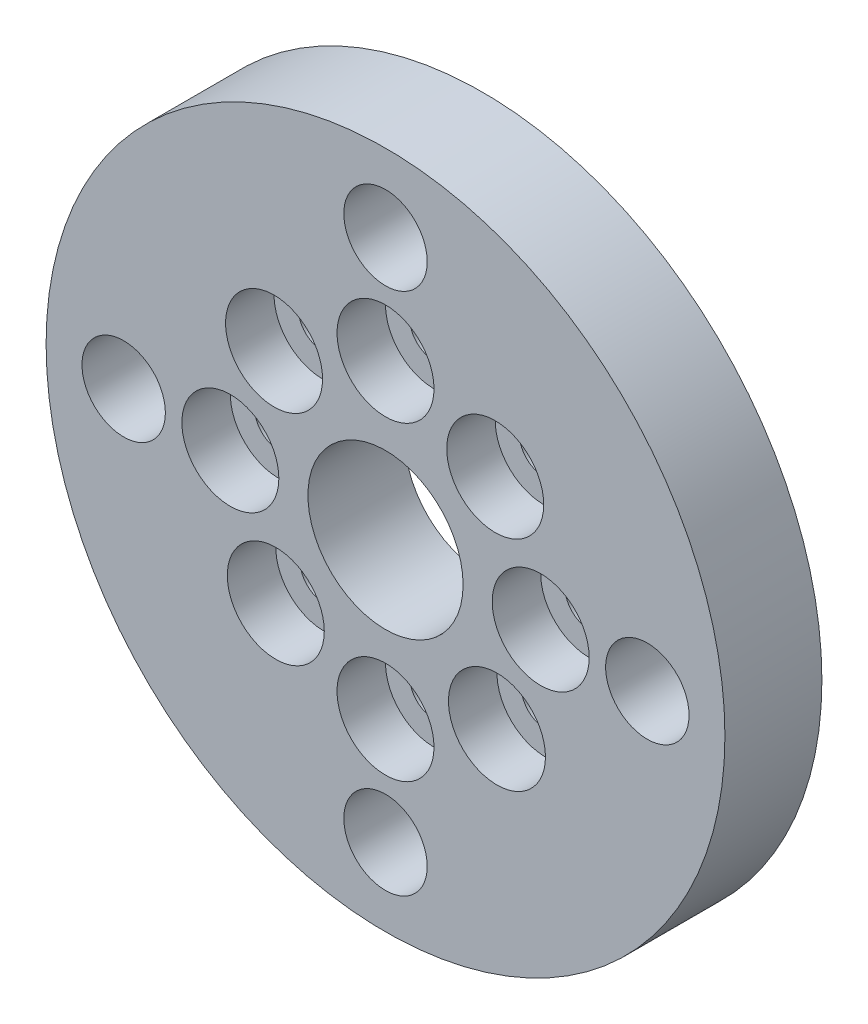
ISO-10303-21;
HEADER;
FILE_DESCRIPTION(('STEP AP214'),'2;1');
FILE_NAME('part.step','',(''),(''),'','','');
FILE_SCHEMA(('AUTOMOTIVE_DESIGN { 1 0 10303 214 1 1 1 1 }'));
ENDSEC;
DATA;
#1=APPLICATION_CONTEXT('core data for automotive mechanical design processes');
#2=APPLICATION_PROTOCOL_DEFINITION('international standard','automotive_design',2000,#1);
#3=PRODUCT_CONTEXT('',#1,'mechanical');
#4=PRODUCT('Part','Part','',(#3));
#5=PRODUCT_RELATED_PRODUCT_CATEGORY('part','',(#4));
#6=PRODUCT_DEFINITION_FORMATION('','',#4);
#7=PRODUCT_DEFINITION_CONTEXT('part definition',#1,'design');
#8=PRODUCT_DEFINITION('design','',#6,#7);
#9=PRODUCT_DEFINITION_SHAPE('','',#8);
#10=(LENGTH_UNIT() NAMED_UNIT(*) SI_UNIT(.MILLI.,.METRE.));
#11=(NAMED_UNIT(*) PLANE_ANGLE_UNIT() SI_UNIT($,.RADIAN.));
#12=(NAMED_UNIT(*) SI_UNIT($,.STERADIAN.) SOLID_ANGLE_UNIT());
#13=UNCERTAINTY_MEASURE_WITH_UNIT(LENGTH_MEASURE(1.E-05),#10,'distance_accuracy_value','');
#14=(GEOMETRIC_REPRESENTATION_CONTEXT(3) GLOBAL_UNCERTAINTY_ASSIGNED_CONTEXT((#13)) GLOBAL_UNIT_ASSIGNED_CONTEXT((#10,
#11,#12)) REPRESENTATION_CONTEXT('',''));
#15=CARTESIAN_POINT('',(0.,0.,0.));
#16=DIRECTION('',(0.,0.,1.));
#17=DIRECTION('',(1.,0.,0.));
#18=AXIS2_PLACEMENT_3D('',#15,#16,#17);
#19=CARTESIAN_POINT('',(0.,0.,10.));
#20=DIRECTION('',(0.,0.,-1.));
#21=DIRECTION('',(-1.,0.,0.));
#22=AXIS2_PLACEMENT_3D('',#19,#20,#21);
#23=CYLINDRICAL_SURFACE('',#22,35.);
#24=CARTESIAN_POINT('',(0.,0.,10.));
#25=DIRECTION('',(0.,0.,1.));
#26=DIRECTION('',(1.,0.,0.));
#27=AXIS2_PLACEMENT_3D('',#24,#25,#26);
#28=CIRCLE('',#27,35.);
#29=CARTESIAN_POINT('',(35.,0.,10.));
#30=VERTEX_POINT('',#29);
#31=EDGE_CURVE('E10',#30,#30,#28,.T.);
#32=ORIENTED_EDGE('',*,*,#31,.F.);
#33=EDGE_LOOP('',(#32));
#34=FACE_BOUND('',#33,.T.);
#35=CARTESIAN_POINT('',(0.,0.,0.));
#36=DIRECTION('',(0.,0.,1.));
#37=DIRECTION('',(1.,0.,0.));
#38=AXIS2_PLACEMENT_3D('',#35,#36,#37);
#39=CIRCLE('',#38,35.);
#40=CARTESIAN_POINT('',(35.,0.,0.));
#41=VERTEX_POINT('',#40);
#42=EDGE_CURVE('E42',#41,#41,#39,.T.);
#43=ORIENTED_EDGE('',*,*,#42,.T.);
#44=EDGE_LOOP('',(#43));
#45=FACE_BOUND('',#44,.T.);
#46=ADVANCED_FACE('F41',(#34,#45),#23,.T.);
#47=CARTESIAN_POINT('',(0.,0.,10.));
#48=DIRECTION('',(0.,0.,1.));
#49=DIRECTION('',(1.,0.,0.));
#50=AXIS2_PLACEMENT_3D('',#47,#48,#49);
#51=PLANE('',#50);
#52=CARTESIAN_POINT('',(11.4925357141582,-11.1320089318505,10.));
#53=DIRECTION('',(0.,0.,1.));
#54=DIRECTION('',(1.,0.,0.));
#55=AXIS2_PLACEMENT_3D('',#52,#53,#54);
#56=CIRCLE('',#55,5.);
#57=CARTESIAN_POINT('',(16.4925357141582,-11.1320089318505,10.));
#58=VERTEX_POINT('',#57);
#59=EDGE_CURVE('E101',#58,#58,#56,.T.);
#60=ORIENTED_EDGE('',*,*,#59,.F.);
#61=EDGE_LOOP('',(#60));
#62=FACE_BOUND('',#61,.T.);
#63=CARTESIAN_POINT('',(-16.,0.,10.));
#64=DIRECTION('',(0.,0.,1.));
#65=DIRECTION('',(1.,0.,0.));
#66=AXIS2_PLACEMENT_3D('',#63,#64,#65);
#67=CIRCLE('',#66,5.);
#68=CARTESIAN_POINT('',(-11.,0.,10.));
#69=VERTEX_POINT('',#68);
#70=EDGE_CURVE('E107',#69,#69,#67,.T.);
#71=ORIENTED_EDGE('',*,*,#70,.F.);
#72=EDGE_LOOP('',(#71));
#73=FACE_BOUND('',#72,.T.);
#74=CARTESIAN_POINT('',(0.,-16.,10.));
#75=DIRECTION('',(0.,0.,1.));
#76=DIRECTION('',(1.,0.,0.));
#77=AXIS2_PLACEMENT_3D('',#74,#75,#76);
#78=CIRCLE('',#77,5.);
#79=CARTESIAN_POINT('',(5.,-16.,10.));
#80=VERTEX_POINT('',#79);
#81=EDGE_CURVE('E90',#80,#80,#78,.T.);
#82=ORIENTED_EDGE('',*,*,#81,.F.);
#83=EDGE_LOOP('',(#82));
#84=FACE_BOUND('',#83,.T.);
#85=CARTESIAN_POINT('',(16.,0.,10.));
#86=DIRECTION('',(0.,0.,1.));
#87=DIRECTION('',(1.,0.,0.));
#88=AXIS2_PLACEMENT_3D('',#85,#86,#87);
#89=CIRCLE('',#88,5.);
#90=CARTESIAN_POINT('',(21.,0.,10.));
#91=VERTEX_POINT('',#90);
#92=EDGE_CURVE('E96',#91,#91,#89,.T.);
#93=ORIENTED_EDGE('',*,*,#92,.F.);
#94=EDGE_LOOP('',(#93));
#95=FACE_BOUND('',#94,.T.);
#96=CARTESIAN_POINT('',(11.3137084989847,11.3137084989848,10.));
#97=DIRECTION('',(0.,0.,1.));
#98=DIRECTION('',(1.,0.,0.));
#99=AXIS2_PLACEMENT_3D('',#96,#97,#98);
#100=CIRCLE('',#99,5.);
#101=CARTESIAN_POINT('',(16.3137084989847,11.3137084989848,10.));
#102=VERTEX_POINT('',#101);
#103=EDGE_CURVE('E127',#102,#102,#100,.T.);
#104=ORIENTED_EDGE('',*,*,#103,.F.);
#105=EDGE_LOOP('',(#104));
#106=FACE_BOUND('',#105,.T.);
#107=CARTESIAN_POINT('',(-11.4925357141582,11.1320089318505,10.));
#108=DIRECTION('',(0.,0.,1.));
#109=DIRECTION('',(1.,0.,0.));
#110=AXIS2_PLACEMENT_3D('',#107,#108,#109);
#111=CIRCLE('',#110,5.);
#112=CARTESIAN_POINT('',(-6.49253571415819,11.1320089318505,10.));
#113=VERTEX_POINT('',#112);
#114=EDGE_CURVE('E116',#113,#113,#111,.T.);
#115=ORIENTED_EDGE('',*,*,#114,.F.);
#116=EDGE_LOOP('',(#115));
#117=FACE_BOUND('',#116,.T.);
#118=CARTESIAN_POINT('',(-11.3137084989847,-11.3137084989848,10.));
#119=DIRECTION('',(0.,0.,1.));
#120=DIRECTION('',(1.,0.,0.));
#121=AXIS2_PLACEMENT_3D('',#118,#119,#120);
#122=CIRCLE('',#121,5.);
#123=CARTESIAN_POINT('',(-6.31370849898474,-11.3137084989848,10.));
#124=VERTEX_POINT('',#123);
#125=EDGE_CURVE('E114',#124,#124,#122,.T.);
#126=ORIENTED_EDGE('',*,*,#125,.F.);
#127=EDGE_LOOP('',(#126));
#128=FACE_BOUND('',#127,.T.);
#129=CARTESIAN_POINT('',(0.,16.,10.));
#130=DIRECTION('',(0.,0.,1.));
#131=DIRECTION('',(1.,0.,0.));
#132=AXIS2_PLACEMENT_3D('',#129,#130,#131);
#133=CIRCLE('',#132,5.);
#134=CARTESIAN_POINT('',(5.,16.,10.));
#135=VERTEX_POINT('',#134);
#136=EDGE_CURVE('E85',#135,#135,#133,.T.);
#137=ORIENTED_EDGE('',*,*,#136,.F.);
#138=EDGE_LOOP('',(#137));
#139=FACE_BOUND('',#138,.T.);
#140=CARTESIAN_POINT('',(0.,27.,10.));
#141=DIRECTION('',(0.,0.,1.));
#142=DIRECTION('',(1.,0.,0.));
#143=AXIS2_PLACEMENT_3D('',#140,#141,#142);
#144=CIRCLE('',#143,4.3);
#145=CARTESIAN_POINT('',(4.3,27.,10.));
#146=VERTEX_POINT('',#145);
#147=EDGE_CURVE('E78',#146,#146,#144,.T.);
#148=ORIENTED_EDGE('',*,*,#147,.F.);
#149=EDGE_LOOP('',(#148));
#150=FACE_BOUND('',#149,.T.);
#151=CARTESIAN_POINT('',(27.,0.,10.));
#152=DIRECTION('',(0.,0.,1.));
#153=DIRECTION('',(1.,0.,0.));
#154=AXIS2_PLACEMENT_3D('',#151,#152,#153);
#155=CIRCLE('',#154,4.3);
#156=CARTESIAN_POINT('',(31.3,0.,10.));
#157=VERTEX_POINT('',#156);
#158=EDGE_CURVE('E75',#157,#157,#155,.T.);
#159=ORIENTED_EDGE('',*,*,#158,.F.);
#160=EDGE_LOOP('',(#159));
#161=FACE_BOUND('',#160,.T.);
#162=CARTESIAN_POINT('',(0.,-27.,10.));
#163=DIRECTION('',(0.,0.,1.));
#164=DIRECTION('',(1.,0.,0.));
#165=AXIS2_PLACEMENT_3D('',#162,#163,#164);
#166=CIRCLE('',#165,4.3);
#167=CARTESIAN_POINT('',(4.3,-27.,10.));
#168=VERTEX_POINT('',#167);
#169=EDGE_CURVE('E67',#168,#168,#166,.T.);
#170=ORIENTED_EDGE('',*,*,#169,.F.);
#171=EDGE_LOOP('',(#170));
#172=FACE_BOUND('',#171,.T.);
#173=CARTESIAN_POINT('',(-27.,0.,10.));
#174=DIRECTION('',(0.,0.,1.));
#175=DIRECTION('',(1.,0.,0.));
#176=AXIS2_PLACEMENT_3D('',#173,#174,#175);
#177=CIRCLE('',#176,4.3);
#178=CARTESIAN_POINT('',(-22.7,0.,10.));
#179=VERTEX_POINT('',#178);
#180=EDGE_CURVE('E56',#179,#179,#177,.T.);
#181=ORIENTED_EDGE('',*,*,#180,.F.);
#182=EDGE_LOOP('',(#181));
#183=FACE_BOUND('',#182,.T.);
#184=CARTESIAN_POINT('',(0.,0.,10.));
#185=DIRECTION('',(0.,0.,1.));
#186=DIRECTION('',(1.,0.,0.));
#187=AXIS2_PLACEMENT_3D('',#184,#185,#186);
#188=CIRCLE('',#187,8.);
#189=CARTESIAN_POINT('',(8.,0.,10.));
#190=VERTEX_POINT('',#189);
#191=EDGE_CURVE('E52',#190,#190,#188,.T.);
#192=ORIENTED_EDGE('',*,*,#191,.F.);
#193=EDGE_LOOP('',(#192));
#194=FACE_BOUND('',#193,.T.);
#195=ORIENTED_EDGE('',*,*,#31,.T.);
#196=EDGE_LOOP('',(#195));
#197=FACE_BOUND('',#196,.T.);
#198=ADVANCED_FACE('F204',(#62,#73,#84,#95,#106,#117,#128,#139,#150,#161,#172,#183,#194,#197),
#51,.T.);
#199=CARTESIAN_POINT('',(0.,0.,0.));
#200=DIRECTION('',(0.,0.,1.));
#201=DIRECTION('',(1.,0.,0.));
#202=AXIS2_PLACEMENT_3D('',#199,#200,#201);
#203=PLANE('',#202);
#204=CARTESIAN_POINT('',(-11.4925357141582,11.1320089318505,0.));
#205=DIRECTION('',(0.,0.,1.));
#206=DIRECTION('',(1.,0.,0.));
#207=AXIS2_PLACEMENT_3D('',#204,#205,#206);
#208=CIRCLE('',#207,2.5);
#209=CARTESIAN_POINT('',(-8.99253571415819,11.1320089318505,0.));
#210=VERTEX_POINT('',#209);
#211=EDGE_CURVE('E138',#210,#210,#208,.T.);
#212=ORIENTED_EDGE('',*,*,#211,.T.);
#213=EDGE_LOOP('',(#212));
#214=FACE_BOUND('',#213,.T.);
#215=CARTESIAN_POINT('',(-16.,0.,0.));
#216=DIRECTION('',(0.,0.,1.));
#217=DIRECTION('',(1.,0.,0.));
#218=AXIS2_PLACEMENT_3D('',#215,#216,#217);
#219=CIRCLE('',#218,2.5);
#220=CARTESIAN_POINT('',(-13.5,0.,0.));
#221=VERTEX_POINT('',#220);
#222=EDGE_CURVE('E148',#221,#221,#219,.T.);
#223=ORIENTED_EDGE('',*,*,#222,.T.);
#224=EDGE_LOOP('',(#223));
#225=FACE_BOUND('',#224,.T.);
#226=CARTESIAN_POINT('',(-11.3137084989847,-11.3137084989848,0.));
#227=DIRECTION('',(0.,0.,1.));
#228=DIRECTION('',(1.,0.,0.));
#229=AXIS2_PLACEMENT_3D('',#226,#227,#228);
#230=CIRCLE('',#229,2.5);
#231=CARTESIAN_POINT('',(-8.81370849898474,-11.3137084989848,0.));
#232=VERTEX_POINT('',#231);
#233=EDGE_CURVE('E155',#232,#232,#230,.T.);
#234=ORIENTED_EDGE('',*,*,#233,.T.);
#235=EDGE_LOOP('',(#234));
#236=FACE_BOUND('',#235,.T.);
#237=CARTESIAN_POINT('',(0.,-16.,0.));
#238=DIRECTION('',(0.,0.,1.));
#239=DIRECTION('',(1.,0.,0.));
#240=AXIS2_PLACEMENT_3D('',#237,#238,#239);
#241=CIRCLE('',#240,2.5);
#242=CARTESIAN_POINT('',(2.5,-16.,0.));
#243=VERTEX_POINT('',#242);
#244=EDGE_CURVE('E158',#243,#243,#241,.T.);
#245=ORIENTED_EDGE('',*,*,#244,.T.);
#246=EDGE_LOOP('',(#245));
#247=FACE_BOUND('',#246,.T.);
#248=CARTESIAN_POINT('',(11.4925357141582,-11.1320089318505,0.));
#249=DIRECTION('',(0.,0.,1.));
#250=DIRECTION('',(1.,0.,0.));
#251=AXIS2_PLACEMENT_3D('',#248,#249,#250);
#252=CIRCLE('',#251,2.5);
#253=CARTESIAN_POINT('',(13.9925357141582,-11.1320089318505,0.));
#254=VERTEX_POINT('',#253);
#255=EDGE_CURVE('E163',#254,#254,#252,.T.);
#256=ORIENTED_EDGE('',*,*,#255,.T.);
#257=EDGE_LOOP('',(#256));
#258=FACE_BOUND('',#257,.T.);
#259=CARTESIAN_POINT('',(16.,0.,0.));
#260=DIRECTION('',(0.,0.,1.));
#261=DIRECTION('',(1.,0.,0.));
#262=AXIS2_PLACEMENT_3D('',#259,#260,#261);
#263=CIRCLE('',#262,2.5);
#264=CARTESIAN_POINT('',(18.5,0.,0.));
#265=VERTEX_POINT('',#264);
#266=EDGE_CURVE('E168',#265,#265,#263,.T.);
#267=ORIENTED_EDGE('',*,*,#266,.T.);
#268=EDGE_LOOP('',(#267));
#269=FACE_BOUND('',#268,.T.);
#270=CARTESIAN_POINT('',(11.3137084989847,11.3137084989848,0.));
#271=DIRECTION('',(0.,0.,1.));
#272=DIRECTION('',(1.,0.,0.));
#273=AXIS2_PLACEMENT_3D('',#270,#271,#272);
#274=CIRCLE('',#273,2.5);
#275=CARTESIAN_POINT('',(13.8137084989847,11.3137084989848,0.));
#276=VERTEX_POINT('',#275);
#277=EDGE_CURVE('E134',#276,#276,#274,.T.);
#278=ORIENTED_EDGE('',*,*,#277,.T.);
#279=EDGE_LOOP('',(#278));
#280=FACE_BOUND('',#279,.T.);
#281=CARTESIAN_POINT('',(0.,16.,0.));
#282=DIRECTION('',(0.,0.,1.));
#283=DIRECTION('',(1.,0.,0.));
#284=AXIS2_PLACEMENT_3D('',#281,#282,#283);
#285=CIRCLE('',#284,2.5);
#286=CARTESIAN_POINT('',(2.5,16.,0.));
#287=VERTEX_POINT('',#286);
#288=EDGE_CURVE('E120',#287,#287,#285,.T.);
#289=ORIENTED_EDGE('',*,*,#288,.T.);
#290=EDGE_LOOP('',(#289));
#291=FACE_BOUND('',#290,.T.);
#292=CARTESIAN_POINT('',(0.,27.,0.));
#293=DIRECTION('',(0.,0.,1.));
#294=DIRECTION('',(1.,0.,0.));
#295=AXIS2_PLACEMENT_3D('',#292,#293,#294);
#296=CIRCLE('',#295,4.3);
#297=CARTESIAN_POINT('',(4.3,27.,0.));
#298=VERTEX_POINT('',#297);
#299=EDGE_CURVE('E57',#298,#298,#296,.T.);
#300=ORIENTED_EDGE('',*,*,#299,.T.);
#301=EDGE_LOOP('',(#300));
#302=FACE_BOUND('',#301,.T.);
#303=CARTESIAN_POINT('',(27.,0.,0.));
#304=DIRECTION('',(0.,0.,1.));
#305=DIRECTION('',(1.,0.,0.));
#306=AXIS2_PLACEMENT_3D('',#303,#304,#305);
#307=CIRCLE('',#306,4.3);
#308=CARTESIAN_POINT('',(31.3,0.,0.));
#309=VERTEX_POINT('',#308);
#310=EDGE_CURVE('E73',#309,#309,#307,.T.);
#311=ORIENTED_EDGE('',*,*,#310,.T.);
#312=EDGE_LOOP('',(#311));
#313=FACE_BOUND('',#312,.T.);
#314=CARTESIAN_POINT('',(0.,-27.,0.));
#315=DIRECTION('',(0.,0.,1.));
#316=DIRECTION('',(1.,0.,0.));
#317=AXIS2_PLACEMENT_3D('',#314,#315,#316);
#318=CIRCLE('',#317,4.3);
#319=CARTESIAN_POINT('',(4.3,-27.,0.));
#320=VERTEX_POINT('',#319);
#321=EDGE_CURVE('E66',#320,#320,#318,.T.);
#322=ORIENTED_EDGE('',*,*,#321,.T.);
#323=EDGE_LOOP('',(#322));
#324=FACE_BOUND('',#323,.T.);
#325=CARTESIAN_POINT('',(-27.,0.,0.));
#326=DIRECTION('',(0.,0.,1.));
#327=DIRECTION('',(1.,0.,0.));
#328=AXIS2_PLACEMENT_3D('',#325,#326,#327);
#329=CIRCLE('',#328,4.3);
#330=CARTESIAN_POINT('',(-22.7,0.,0.));
#331=VERTEX_POINT('',#330);
#332=EDGE_CURVE('E65',#331,#331,#329,.T.);
#333=ORIENTED_EDGE('',*,*,#332,.T.);
#334=EDGE_LOOP('',(#333));
#335=FACE_BOUND('',#334,.T.);
#336=CARTESIAN_POINT('',(0.,0.,0.));
#337=DIRECTION('',(0.,0.,1.));
#338=DIRECTION('',(1.,0.,0.));
#339=AXIS2_PLACEMENT_3D('',#336,#337,#338);
#340=CIRCLE('',#339,8.);
#341=CARTESIAN_POINT('',(8.,0.,0.));
#342=VERTEX_POINT('',#341);
#343=EDGE_CURVE('E51',#342,#342,#340,.T.);
#344=ORIENTED_EDGE('',*,*,#343,.T.);
#345=EDGE_LOOP('',(#344));
#346=FACE_BOUND('',#345,.T.);
#347=ORIENTED_EDGE('',*,*,#42,.F.);
#348=EDGE_LOOP('',(#347));
#349=FACE_BOUND('',#348,.T.);
#350=ADVANCED_FACE('F176',(#214,#225,#236,#247,#258,#269,#280,#291,#302,#313,#324,#335,#346,
#349),#203,.F.);
#351=CARTESIAN_POINT('',(0.,0.,0.));
#352=DIRECTION('',(0.,0.,1.));
#353=DIRECTION('',(1.,0.,0.));
#354=AXIS2_PLACEMENT_3D('',#351,#352,#353);
#355=CYLINDRICAL_SURFACE('',#354,8.);
#356=ORIENTED_EDGE('',*,*,#343,.F.);
#357=EDGE_LOOP('',(#356));
#358=FACE_BOUND('',#357,.T.);
#359=ORIENTED_EDGE('',*,*,#191,.T.);
#360=EDGE_LOOP('',(#359));
#361=FACE_BOUND('',#360,.T.);
#362=ADVANCED_FACE('F223',(#358,#361),#355,.F.);
#363=CARTESIAN_POINT('',(-27.,0.,0.));
#364=DIRECTION('',(0.,0.,1.));
#365=DIRECTION('',(1.,0.,0.));
#366=AXIS2_PLACEMENT_3D('',#363,#364,#365);
#367=CYLINDRICAL_SURFACE('',#366,4.3);
#368=ORIENTED_EDGE('',*,*,#332,.F.);
#369=EDGE_LOOP('',(#368));
#370=FACE_BOUND('',#369,.T.);
#371=ORIENTED_EDGE('',*,*,#180,.T.);
#372=EDGE_LOOP('',(#371));
#373=FACE_BOUND('',#372,.T.);
#374=ADVANCED_FACE('F230',(#370,#373),#367,.F.);
#375=CARTESIAN_POINT('',(0.,-27.,0.));
#376=DIRECTION('',(0.,0.,1.));
#377=DIRECTION('',(1.,0.,0.));
#378=AXIS2_PLACEMENT_3D('',#375,#376,#377);
#379=CYLINDRICAL_SURFACE('',#378,4.3);
#380=ORIENTED_EDGE('',*,*,#321,.F.);
#381=EDGE_LOOP('',(#380));
#382=FACE_BOUND('',#381,.T.);
#383=ORIENTED_EDGE('',*,*,#169,.T.);
#384=EDGE_LOOP('',(#383));
#385=FACE_BOUND('',#384,.T.);
#386=ADVANCED_FACE('F231',(#382,#385),#379,.F.);
#387=CARTESIAN_POINT('',(27.,0.,0.));
#388=DIRECTION('',(0.,0.,1.));
#389=DIRECTION('',(1.,0.,0.));
#390=AXIS2_PLACEMENT_3D('',#387,#388,#389);
#391=CYLINDRICAL_SURFACE('',#390,4.3);
#392=ORIENTED_EDGE('',*,*,#310,.F.);
#393=EDGE_LOOP('',(#392));
#394=FACE_BOUND('',#393,.T.);
#395=ORIENTED_EDGE('',*,*,#158,.T.);
#396=EDGE_LOOP('',(#395));
#397=FACE_BOUND('',#396,.T.);
#398=ADVANCED_FACE('F274',(#394,#397),#391,.F.);
#399=CARTESIAN_POINT('',(0.,27.,0.));
#400=DIRECTION('',(0.,0.,1.));
#401=DIRECTION('',(1.,0.,0.));
#402=AXIS2_PLACEMENT_3D('',#399,#400,#401);
#403=CYLINDRICAL_SURFACE('',#402,4.3);
#404=ORIENTED_EDGE('',*,*,#299,.F.);
#405=EDGE_LOOP('',(#404));
#406=FACE_BOUND('',#405,.T.);
#407=ORIENTED_EDGE('',*,*,#147,.T.);
#408=EDGE_LOOP('',(#407));
#409=FACE_BOUND('',#408,.T.);
#410=ADVANCED_FACE('F281',(#406,#409),#403,.F.);
#411=CARTESIAN_POINT('',(0.,16.,5.));
#412=DIRECTION('',(0.,0.,1.));
#413=DIRECTION('',(1.,0.,0.));
#414=AXIS2_PLACEMENT_3D('',#411,#412,#413);
#415=CYLINDRICAL_SURFACE('',#414,5.);
#416=CARTESIAN_POINT('',(0.,16.,5.));
#417=DIRECTION('',(0.,0.,1.));
#418=DIRECTION('',(1.,0.,0.));
#419=AXIS2_PLACEMENT_3D('',#416,#417,#418);
#420=CIRCLE('',#419,5.);
#421=CARTESIAN_POINT('',(5.,16.,5.));
#422=VERTEX_POINT('',#421);
#423=EDGE_CURVE('E63',#422,#422,#420,.T.);
#424=ORIENTED_EDGE('',*,*,#423,.F.);
#425=EDGE_LOOP('',(#424));
#426=FACE_BOUND('',#425,.T.);
#427=ORIENTED_EDGE('',*,*,#136,.T.);
#428=EDGE_LOOP('',(#427));
#429=FACE_BOUND('',#428,.T.);
#430=ADVANCED_FACE('F293',(#426,#429),#415,.F.);
#431=CARTESIAN_POINT('',(0.,16.,5.));
#432=DIRECTION('',(0.,0.,1.));
#433=DIRECTION('',(1.,0.,0.));
#434=AXIS2_PLACEMENT_3D('',#431,#432,#433);
#435=PLANE('',#434);
#436=CARTESIAN_POINT('',(0.,16.,5.));
#437=DIRECTION('',(0.,0.,1.));
#438=DIRECTION('',(1.,0.,0.));
#439=AXIS2_PLACEMENT_3D('',#436,#437,#438);
#440=CIRCLE('',#439,2.5);
#441=CARTESIAN_POINT('',(2.5,16.,5.));
#442=VERTEX_POINT('',#441);
#443=EDGE_CURVE('E132',#442,#442,#440,.T.);
#444=ORIENTED_EDGE('',*,*,#443,.F.);
#445=EDGE_LOOP('',(#444));
#446=FACE_BOUND('',#445,.T.);
#447=ORIENTED_EDGE('',*,*,#423,.T.);
#448=EDGE_LOOP('',(#447));
#449=FACE_BOUND('',#448,.T.);
#450=ADVANCED_FACE('F303',(#446,#449),#435,.T.);
#451=CARTESIAN_POINT('',(-11.3137084989847,-11.3137084989848,5.));
#452=DIRECTION('',(0.,0.,1.));
#453=DIRECTION('',(1.,0.,0.));
#454=AXIS2_PLACEMENT_3D('',#451,#452,#453);
#455=CYLINDRICAL_SURFACE('',#454,5.);
#456=CARTESIAN_POINT('',(-11.3137084989847,-11.3137084989848,5.));
#457=DIRECTION('',(0.,0.,1.));
#458=DIRECTION('',(1.,0.,0.));
#459=AXIS2_PLACEMENT_3D('',#456,#457,#458);
#460=CIRCLE('',#459,5.);
#461=CARTESIAN_POINT('',(-6.31370849898474,-11.3137084989848,5.));
#462=VERTEX_POINT('',#461);
#463=EDGE_CURVE('E117',#462,#462,#460,.T.);
#464=ORIENTED_EDGE('',*,*,#463,.F.);
#465=EDGE_LOOP('',(#464));
#466=FACE_BOUND('',#465,.T.);
#467=ORIENTED_EDGE('',*,*,#125,.T.);
#468=EDGE_LOOP('',(#467));
#469=FACE_BOUND('',#468,.T.);
#470=ADVANCED_FACE('F312',(#466,#469),#455,.F.);
#471=CARTESIAN_POINT('',(-11.3137084989847,-11.3137084989848,5.));
#472=DIRECTION('',(0.,0.,1.));
#473=DIRECTION('',(1.,0.,0.));
#474=AXIS2_PLACEMENT_3D('',#471,#472,#473);
#475=PLANE('',#474);
#476=CARTESIAN_POINT('',(-11.3137084989847,-11.3137084989848,5.));
#477=DIRECTION('',(0.,0.,1.));
#478=DIRECTION('',(1.,0.,0.));
#479=AXIS2_PLACEMENT_3D('',#476,#477,#478);
#480=CIRCLE('',#479,2.5);
#481=CARTESIAN_POINT('',(-8.81370849898474,-11.3137084989848,5.));
#482=VERTEX_POINT('',#481);
#483=EDGE_CURVE('E149',#482,#482,#480,.T.);
#484=ORIENTED_EDGE('',*,*,#483,.F.);
#485=EDGE_LOOP('',(#484));
#486=FACE_BOUND('',#485,.T.);
#487=ORIENTED_EDGE('',*,*,#463,.T.);
#488=EDGE_LOOP('',(#487));
#489=FACE_BOUND('',#488,.T.);
#490=ADVANCED_FACE('F324',(#486,#489),#475,.T.);
#491=CARTESIAN_POINT('',(-11.4925357141582,11.1320089318505,5.));
#492=DIRECTION('',(0.,0.,1.));
#493=DIRECTION('',(1.,0.,0.));
#494=AXIS2_PLACEMENT_3D('',#491,#492,#493);
#495=CYLINDRICAL_SURFACE('',#494,5.);
#496=CARTESIAN_POINT('',(-11.4925357141582,11.1320089318505,5.));
#497=DIRECTION('',(0.,0.,1.));
#498=DIRECTION('',(1.,0.,0.));
#499=AXIS2_PLACEMENT_3D('',#496,#497,#498);
#500=CIRCLE('',#499,5.);
#501=CARTESIAN_POINT('',(-6.49253571415819,11.1320089318505,5.));
#502=VERTEX_POINT('',#501);
#503=EDGE_CURVE('E125',#502,#502,#500,.T.);
#504=ORIENTED_EDGE('',*,*,#503,.F.);
#505=EDGE_LOOP('',(#504));
#506=FACE_BOUND('',#505,.T.);
#507=ORIENTED_EDGE('',*,*,#114,.T.);
#508=EDGE_LOOP('',(#507));
#509=FACE_BOUND('',#508,.T.);
#510=ADVANCED_FACE('F333',(#506,#509),#495,.F.);
#511=CARTESIAN_POINT('',(-11.4925357141582,11.1320089318505,5.));
#512=DIRECTION('',(0.,0.,1.));
#513=DIRECTION('',(1.,0.,0.));
#514=AXIS2_PLACEMENT_3D('',#511,#512,#513);
#515=PLANE('',#514);
#516=CARTESIAN_POINT('',(-11.4925357141582,11.1320089318505,5.));
#517=DIRECTION('',(0.,0.,1.));
#518=DIRECTION('',(1.,0.,0.));
#519=AXIS2_PLACEMENT_3D('',#516,#517,#518);
#520=CIRCLE('',#519,2.5);
#521=CARTESIAN_POINT('',(-8.99253571415819,11.1320089318505,5.));
#522=VERTEX_POINT('',#521);
#523=EDGE_CURVE('E139',#522,#522,#520,.T.);
#524=ORIENTED_EDGE('',*,*,#523,.F.);
#525=EDGE_LOOP('',(#524));
#526=FACE_BOUND('',#525,.T.);
#527=ORIENTED_EDGE('',*,*,#503,.T.);
#528=EDGE_LOOP('',(#527));
#529=FACE_BOUND('',#528,.T.);
#530=ADVANCED_FACE('F199',(#526,#529),#515,.T.);
#531=CARTESIAN_POINT('',(11.3137084989847,11.3137084989848,5.));
#532=DIRECTION('',(0.,0.,1.));
#533=DIRECTION('',(1.,0.,0.));
#534=AXIS2_PLACEMENT_3D('',#531,#532,#533);
#535=CYLINDRICAL_SURFACE('',#534,5.);
#536=CARTESIAN_POINT('',(11.3137084989847,11.3137084989848,5.));
#537=DIRECTION('',(0.,0.,1.));
#538=DIRECTION('',(1.,0.,0.));
#539=AXIS2_PLACEMENT_3D('',#536,#537,#538);
#540=CIRCLE('',#539,5.);
#541=CARTESIAN_POINT('',(16.3137084989847,11.3137084989848,5.));
#542=VERTEX_POINT('',#541);
#543=EDGE_CURVE('E104',#542,#542,#540,.T.);
#544=ORIENTED_EDGE('',*,*,#543,.F.);
#545=EDGE_LOOP('',(#544));
#546=FACE_BOUND('',#545,.T.);
#547=ORIENTED_EDGE('',*,*,#103,.T.);
#548=EDGE_LOOP('',(#547));
#549=FACE_BOUND('',#548,.T.);
#550=ADVANCED_FACE('F191',(#546,#549),#535,.F.);
#551=CARTESIAN_POINT('',(11.3137084989847,11.3137084989848,5.));
#552=DIRECTION('',(0.,0.,1.));
#553=DIRECTION('',(1.,0.,0.));
#554=AXIS2_PLACEMENT_3D('',#551,#552,#553);
#555=PLANE('',#554);
#556=CARTESIAN_POINT('',(11.3137084989847,11.3137084989848,5.));
#557=DIRECTION('',(0.,0.,1.));
#558=DIRECTION('',(1.,0.,0.));
#559=AXIS2_PLACEMENT_3D('',#556,#557,#558);
#560=CIRCLE('',#559,2.5);
#561=CARTESIAN_POINT('',(13.8137084989847,11.3137084989848,5.));
#562=VERTEX_POINT('',#561);
#563=EDGE_CURVE('E173',#562,#562,#560,.T.);
#564=ORIENTED_EDGE('',*,*,#563,.F.);
#565=EDGE_LOOP('',(#564));
#566=FACE_BOUND('',#565,.T.);
#567=ORIENTED_EDGE('',*,*,#543,.T.);
#568=EDGE_LOOP('',(#567));
#569=FACE_BOUND('',#568,.T.);
#570=ADVANCED_FACE('F186',(#566,#569),#555,.T.);
#571=CARTESIAN_POINT('',(16.,0.,5.));
#572=DIRECTION('',(0.,0.,1.));
#573=DIRECTION('',(1.,0.,0.));
#574=AXIS2_PLACEMENT_3D('',#571,#572,#573);
#575=CYLINDRICAL_SURFACE('',#574,5.);
#576=CARTESIAN_POINT('',(16.,0.,5.));
#577=DIRECTION('',(0.,0.,1.));
#578=DIRECTION('',(1.,0.,0.));
#579=AXIS2_PLACEMENT_3D('',#576,#577,#578);
#580=CIRCLE('',#579,5.);
#581=CARTESIAN_POINT('',(21.,0.,5.));
#582=VERTEX_POINT('',#581);
#583=EDGE_CURVE('E88',#582,#582,#580,.T.);
#584=ORIENTED_EDGE('',*,*,#583,.F.);
#585=EDGE_LOOP('',(#584));
#586=FACE_BOUND('',#585,.T.);
#587=ORIENTED_EDGE('',*,*,#92,.T.);
#588=EDGE_LOOP('',(#587));
#589=FACE_BOUND('',#588,.T.);
#590=ADVANCED_FACE('F195',(#586,#589),#575,.F.);
#591=CARTESIAN_POINT('',(16.,0.,5.));
#592=DIRECTION('',(0.,0.,1.));
#593=DIRECTION('',(1.,0.,0.));
#594=AXIS2_PLACEMENT_3D('',#591,#592,#593);
#595=PLANE('',#594);
#596=CARTESIAN_POINT('',(16.,0.,5.));
#597=DIRECTION('',(0.,0.,1.));
#598=DIRECTION('',(1.,0.,0.));
#599=AXIS2_PLACEMENT_3D('',#596,#597,#598);
#600=CIRCLE('',#599,2.5);
#601=CARTESIAN_POINT('',(18.5,0.,5.));
#602=VERTEX_POINT('',#601);
#603=EDGE_CURVE('E170',#602,#602,#600,.T.);
#604=ORIENTED_EDGE('',*,*,#603,.F.);
#605=EDGE_LOOP('',(#604));
#606=FACE_BOUND('',#605,.T.);
#607=ORIENTED_EDGE('',*,*,#583,.T.);
#608=EDGE_LOOP('',(#607));
#609=FACE_BOUND('',#608,.T.);
#610=ADVANCED_FACE('F374',(#606,#609),#595,.T.);
#611=CARTESIAN_POINT('',(0.,-16.,5.));
#612=DIRECTION('',(0.,0.,1.));
#613=DIRECTION('',(1.,0.,0.));
#614=AXIS2_PLACEMENT_3D('',#611,#612,#613);
#615=CYLINDRICAL_SURFACE('',#614,5.);
#616=CARTESIAN_POINT('',(0.,-16.,5.));
#617=DIRECTION('',(0.,0.,1.));
#618=DIRECTION('',(1.,0.,0.));
#619=AXIS2_PLACEMENT_3D('',#616,#617,#618);
#620=CIRCLE('',#619,5.);
#621=CARTESIAN_POINT('',(5.,-16.,5.));
#622=VERTEX_POINT('',#621);
#623=EDGE_CURVE('E95',#622,#622,#620,.T.);
#624=ORIENTED_EDGE('',*,*,#623,.F.);
#625=EDGE_LOOP('',(#624));
#626=FACE_BOUND('',#625,.T.);
#627=ORIENTED_EDGE('',*,*,#81,.T.);
#628=EDGE_LOOP('',(#627));
#629=FACE_BOUND('',#628,.T.);
#630=ADVANCED_FACE('F384',(#626,#629),#615,.F.);
#631=CARTESIAN_POINT('',(0.,-16.,5.));
#632=DIRECTION('',(0.,0.,1.));
#633=DIRECTION('',(1.,0.,0.));
#634=AXIS2_PLACEMENT_3D('',#631,#632,#633);
#635=PLANE('',#634);
#636=CARTESIAN_POINT('',(0.,-16.,5.));
#637=DIRECTION('',(0.,0.,1.));
#638=DIRECTION('',(1.,0.,0.));
#639=AXIS2_PLACEMENT_3D('',#636,#637,#638);
#640=CIRCLE('',#639,2.5);
#641=CARTESIAN_POINT('',(2.5,-16.,5.));
#642=VERTEX_POINT('',#641);
#643=EDGE_CURVE('E154',#642,#642,#640,.T.);
#644=ORIENTED_EDGE('',*,*,#643,.F.);
#645=EDGE_LOOP('',(#644));
#646=FACE_BOUND('',#645,.T.);
#647=ORIENTED_EDGE('',*,*,#623,.T.);
#648=EDGE_LOOP('',(#647));
#649=FACE_BOUND('',#648,.T.);
#650=ADVANCED_FACE('F391',(#646,#649),#635,.T.);
#651=CARTESIAN_POINT('',(-16.,0.,5.));
#652=DIRECTION('',(0.,0.,1.));
#653=DIRECTION('',(1.,0.,0.));
#654=AXIS2_PLACEMENT_3D('',#651,#652,#653);
#655=CYLINDRICAL_SURFACE('',#654,5.);
#656=CARTESIAN_POINT('',(-16.,0.,5.));
#657=DIRECTION('',(0.,0.,1.));
#658=DIRECTION('',(1.,0.,0.));
#659=AXIS2_PLACEMENT_3D('',#656,#657,#658);
#660=CIRCLE('',#659,5.);
#661=CARTESIAN_POINT('',(-11.,0.,5.));
#662=VERTEX_POINT('',#661);
#663=EDGE_CURVE('E91',#662,#662,#660,.T.);
#664=ORIENTED_EDGE('',*,*,#663,.F.);
#665=EDGE_LOOP('',(#664));
#666=FACE_BOUND('',#665,.T.);
#667=ORIENTED_EDGE('',*,*,#70,.T.);
#668=EDGE_LOOP('',(#667));
#669=FACE_BOUND('',#668,.T.);
#670=ADVANCED_FACE('F403',(#666,#669),#655,.F.);
#671=CARTESIAN_POINT('',(-16.,0.,5.));
#672=DIRECTION('',(0.,0.,1.));
#673=DIRECTION('',(1.,0.,0.));
#674=AXIS2_PLACEMENT_3D('',#671,#672,#673);
#675=PLANE('',#674);
#676=CARTESIAN_POINT('',(-16.,0.,5.));
#677=DIRECTION('',(0.,0.,1.));
#678=DIRECTION('',(1.,0.,0.));
#679=AXIS2_PLACEMENT_3D('',#676,#677,#678);
#680=CIRCLE('',#679,2.5);
#681=CARTESIAN_POINT('',(-13.5,0.,5.));
#682=VERTEX_POINT('',#681);
#683=EDGE_CURVE('E141',#682,#682,#680,.T.);
#684=ORIENTED_EDGE('',*,*,#683,.F.);
#685=EDGE_LOOP('',(#684));
#686=FACE_BOUND('',#685,.T.);
#687=ORIENTED_EDGE('',*,*,#663,.T.);
#688=EDGE_LOOP('',(#687));
#689=FACE_BOUND('',#688,.T.);
#690=ADVANCED_FACE('F413',(#686,#689),#675,.T.);
#691=CARTESIAN_POINT('',(11.4925357141582,-11.1320089318505,5.));
#692=DIRECTION('',(0.,0.,1.));
#693=DIRECTION('',(1.,0.,0.));
#694=AXIS2_PLACEMENT_3D('',#691,#692,#693);
#695=CYLINDRICAL_SURFACE('',#694,5.);
#696=CARTESIAN_POINT('',(11.4925357141582,-11.1320089318505,5.));
#697=DIRECTION('',(0.,0.,1.));
#698=DIRECTION('',(1.,0.,0.));
#699=AXIS2_PLACEMENT_3D('',#696,#697,#698);
#700=CIRCLE('',#699,5.);
#701=CARTESIAN_POINT('',(16.4925357141582,-11.1320089318505,5.));
#702=VERTEX_POINT('',#701);
#703=EDGE_CURVE('E102',#702,#702,#700,.T.);
#704=ORIENTED_EDGE('',*,*,#703,.F.);
#705=EDGE_LOOP('',(#704));
#706=FACE_BOUND('',#705,.T.);
#707=ORIENTED_EDGE('',*,*,#59,.T.);
#708=EDGE_LOOP('',(#707));
#709=FACE_BOUND('',#708,.T.);
#710=ADVANCED_FACE('F424',(#706,#709),#695,.F.);
#711=CARTESIAN_POINT('',(11.4925357141582,-11.1320089318505,5.));
#712=DIRECTION('',(0.,0.,1.));
#713=DIRECTION('',(1.,0.,0.));
#714=AXIS2_PLACEMENT_3D('',#711,#712,#713);
#715=PLANE('',#714);
#716=CARTESIAN_POINT('',(11.4925357141582,-11.1320089318505,5.));
#717=DIRECTION('',(0.,0.,1.));
#718=DIRECTION('',(1.,0.,0.));
#719=AXIS2_PLACEMENT_3D('',#716,#717,#718);
#720=CIRCLE('',#719,2.5);
#721=CARTESIAN_POINT('',(13.9925357141582,-11.1320089318505,5.));
#722=VERTEX_POINT('',#721);
#723=EDGE_CURVE('E161',#722,#722,#720,.T.);
#724=ORIENTED_EDGE('',*,*,#723,.F.);
#725=EDGE_LOOP('',(#724));
#726=FACE_BOUND('',#725,.T.);
#727=ORIENTED_EDGE('',*,*,#703,.T.);
#728=EDGE_LOOP('',(#727));
#729=FACE_BOUND('',#728,.T.);
#730=ADVANCED_FACE('F432',(#726,#729),#715,.T.);
#731=CARTESIAN_POINT('',(0.,16.,0.));
#732=DIRECTION('',(0.,0.,1.));
#733=DIRECTION('',(1.,0.,0.));
#734=AXIS2_PLACEMENT_3D('',#731,#732,#733);
#735=CYLINDRICAL_SURFACE('',#734,2.5);
#736=ORIENTED_EDGE('',*,*,#288,.F.);
#737=EDGE_LOOP('',(#736));
#738=FACE_BOUND('',#737,.T.);
#739=ORIENTED_EDGE('',*,*,#443,.T.);
#740=EDGE_LOOP('',(#739));
#741=FACE_BOUND('',#740,.T.);
#742=ADVANCED_FACE('F187',(#738,#741),#735,.F.);
#743=CARTESIAN_POINT('',(11.3137084989847,11.3137084989848,0.));
#744=DIRECTION('',(0.,0.,1.));
#745=DIRECTION('',(1.,0.,0.));
#746=AXIS2_PLACEMENT_3D('',#743,#744,#745);
#747=CYLINDRICAL_SURFACE('',#746,2.5);
#748=ORIENTED_EDGE('',*,*,#277,.F.);
#749=EDGE_LOOP('',(#748));
#750=FACE_BOUND('',#749,.T.);
#751=ORIENTED_EDGE('',*,*,#563,.T.);
#752=EDGE_LOOP('',(#751));
#753=FACE_BOUND('',#752,.T.);
#754=ADVANCED_FACE('F185',(#750,#753),#747,.F.);
#755=CARTESIAN_POINT('',(16.,0.,0.));
#756=DIRECTION('',(0.,0.,1.));
#757=DIRECTION('',(1.,0.,0.));
#758=AXIS2_PLACEMENT_3D('',#755,#756,#757);
#759=CYLINDRICAL_SURFACE('',#758,2.5);
#760=ORIENTED_EDGE('',*,*,#266,.F.);
#761=EDGE_LOOP('',(#760));
#762=FACE_BOUND('',#761,.T.);
#763=ORIENTED_EDGE('',*,*,#603,.T.);
#764=EDGE_LOOP('',(#763));
#765=FACE_BOUND('',#764,.T.);
#766=ADVANCED_FACE('F183',(#762,#765),#759,.F.);
#767=CARTESIAN_POINT('',(11.4925357141582,-11.1320089318505,0.));
#768=DIRECTION('',(0.,0.,1.));
#769=DIRECTION('',(1.,0.,0.));
#770=AXIS2_PLACEMENT_3D('',#767,#768,#769);
#771=CYLINDRICAL_SURFACE('',#770,2.5);
#772=ORIENTED_EDGE('',*,*,#255,.F.);
#773=EDGE_LOOP('',(#772));
#774=FACE_BOUND('',#773,.T.);
#775=ORIENTED_EDGE('',*,*,#723,.T.);
#776=EDGE_LOOP('',(#775));
#777=FACE_BOUND('',#776,.T.);
#778=ADVANCED_FACE('F469',(#774,#777),#771,.F.);
#779=CARTESIAN_POINT('',(0.,-16.,0.));
#780=DIRECTION('',(0.,0.,1.));
#781=DIRECTION('',(1.,0.,0.));
#782=AXIS2_PLACEMENT_3D('',#779,#780,#781);
#783=CYLINDRICAL_SURFACE('',#782,2.5);
#784=ORIENTED_EDGE('',*,*,#244,.F.);
#785=EDGE_LOOP('',(#784));
#786=FACE_BOUND('',#785,.T.);
#787=ORIENTED_EDGE('',*,*,#643,.T.);
#788=EDGE_LOOP('',(#787));
#789=FACE_BOUND('',#788,.T.);
#790=ADVANCED_FACE('F480',(#786,#789),#783,.F.);
#791=CARTESIAN_POINT('',(-11.3137084989847,-11.3137084989848,0.));
#792=DIRECTION('',(0.,0.,1.));
#793=DIRECTION('',(1.,0.,0.));
#794=AXIS2_PLACEMENT_3D('',#791,#792,#793);
#795=CYLINDRICAL_SURFACE('',#794,2.5);
#796=ORIENTED_EDGE('',*,*,#233,.F.);
#797=EDGE_LOOP('',(#796));
#798=FACE_BOUND('',#797,.T.);
#799=ORIENTED_EDGE('',*,*,#483,.T.);
#800=EDGE_LOOP('',(#799));
#801=FACE_BOUND('',#800,.T.);
#802=ADVANCED_FACE('F490',(#798,#801),#795,.F.);
#803=CARTESIAN_POINT('',(-16.,0.,0.));
#804=DIRECTION('',(0.,0.,1.));
#805=DIRECTION('',(1.,0.,0.));
#806=AXIS2_PLACEMENT_3D('',#803,#804,#805);
#807=CYLINDRICAL_SURFACE('',#806,2.5);
#808=ORIENTED_EDGE('',*,*,#222,.F.);
#809=EDGE_LOOP('',(#808));
#810=FACE_BOUND('',#809,.T.);
#811=ORIENTED_EDGE('',*,*,#683,.T.);
#812=EDGE_LOOP('',(#811));
#813=FACE_BOUND('',#812,.T.);
#814=ADVANCED_FACE('F500',(#810,#813),#807,.F.);
#815=CARTESIAN_POINT('',(-11.4925357141582,11.1320089318505,0.));
#816=DIRECTION('',(0.,0.,1.));
#817=DIRECTION('',(1.,0.,0.));
#818=AXIS2_PLACEMENT_3D('',#815,#816,#817);
#819=CYLINDRICAL_SURFACE('',#818,2.5);
#820=ORIENTED_EDGE('',*,*,#211,.F.);
#821=EDGE_LOOP('',(#820));
#822=FACE_BOUND('',#821,.T.);
#823=ORIENTED_EDGE('',*,*,#523,.T.);
#824=EDGE_LOOP('',(#823));
#825=FACE_BOUND('',#824,.T.);
#826=ADVANCED_FACE('F509',(#822,#825),#819,.F.);
#827=CLOSED_SHELL('',(#46,#198,#350,#362,#374,#386,#398,#410,#430,#450,#470,#490,#510,#530,#550,
#570,#590,#610,#630,#650,#670,#690,#710,#730,#742,#754,#766,#778,#790,#802,#814,#826));
#828=MANIFOLD_SOLID_BREP('B2',#827);
#829=ADVANCED_BREP_SHAPE_REPRESENTATION('',(#18,#828),#14);
#830=SHAPE_DEFINITION_REPRESENTATION(#9,#829);
ENDSEC;
END-ISO-10303-21;
